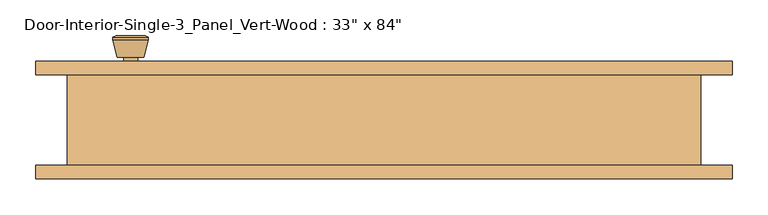
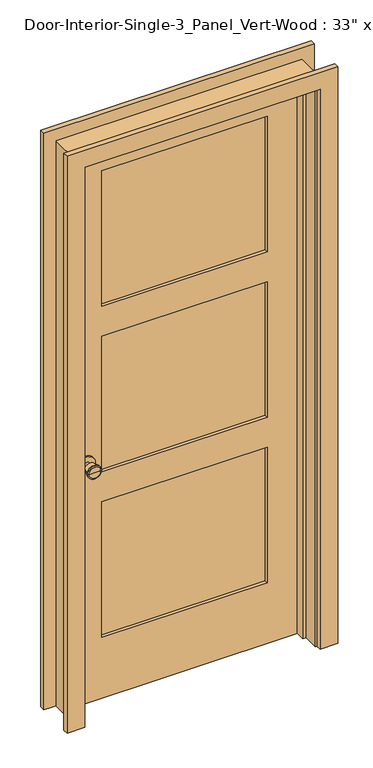
"""IFC4 building model written with IfcOpenShell, lengths in millimetres: door geometry."""

from ifc_helpers import new_model, si_unit, point, frame, frame_2d, origin, place, context, project, spatial, polyline, circle_curve, trimmed, segment, composite_curve, outline, extrude, faceted_brep, source, transform, mapped, element, save
from ifc_brep_helpers import plane_surface, cylinder_surface, revolved_surface, advanced_brep


def door_14766595(model_context):
    return source(origin(), model_context, "Body", "SolidModel", [
        advanced_brep(
        [(-355.6, 19.4, 914.4), (-345.6, 19.4, 914.4), (-365.6, 19.4, 914.4), (-335.1241324, -29.6, 914.4), (-355.6, -29.6, 914.4), (-376.0758676, -29.6, 914.4), (-330.6, -27.7721319, 914.4), (-380.6, -27.7721319, 914.4), (-330.6, -24.3084537, 914.4), (-380.6, -24.3084537, 914.4), (-336.963764, 0.4, 914.4), (-374.236236, 0.4, 914.4), (-345.6, 0.4, 914.4), (-365.6, 0.4, 914.4)],
        [
            (0, 1),
            (1, 2, circle_curve(frame((-355.6, 19.4, 914.4), z_axis=(0.0, 1.0, 0.0), x_axis=(-1.0, 0.0, 0.0)), 10.0)),
            (2, 0),
            (2, 1, circle_curve(frame((-355.6, 19.4, 914.4), z_axis=(0.0, 1.0, 0.0), x_axis=(-1.0, 0.0, 0.0)), 10.0)),
            (3, 4),
            (4, 5),
            (5, 3, circle_curve(frame((-355.6, -29.6, 914.4), z_axis=(0.0, -1.0, 0.0), x_axis=(-1.0, 0.0, 0.0)), 20.4758676)),
            (3, 5, circle_curve(frame((-355.6, -29.6, 914.4), z_axis=(0.0, -1.0, 0.0), x_axis=(-1.0, 0.0, 0.0)), 20.4758676)),
            (6, 3),
            (5, 7),
            (7, 6, circle_curve(frame((-355.6, -27.7721319, 914.4), z_axis=(0.0, -1.0, 0.0), x_axis=(-1.0, 0.0, 0.0)), 25.0)),
            (6, 7, circle_curve(frame((-355.6, -27.7721319, 914.4), z_axis=(0.0, -1.0, 0.0), x_axis=(-1.0, 0.0, 0.0)), 25.0)),
            (8, 6),
            (7, 9),
            (9, 8, circle_curve(frame((-355.6, -24.3084537, 914.4), z_axis=(0.0, -1.0, 0.0), x_axis=(-1.0, 0.0, 0.0)), 25.0)),
            (8, 9, circle_curve(frame((-355.6, -24.3084537, 914.4), z_axis=(0.0, -1.0, 0.0), x_axis=(-1.0, 0.0, 0.0)), 25.0)),
            (10, 8),
            (9, 11),
            (11, 10, circle_curve(frame((-355.6, 0.4, 914.4), z_axis=(0.0, -1.0, 0.0), x_axis=(-1.0, 0.0, 0.0)), 18.636236)),
            (10, 11, circle_curve(frame((-355.6, 0.4, 914.4), z_axis=(0.0, -1.0, 0.0), x_axis=(-1.0, 0.0, 0.0)), 18.636236)),
            (12, 10),
            (11, 13),
            (13, 12, circle_curve(frame((-355.6, 0.4, 914.4), z_axis=(0.0, -1.0, 0.0), x_axis=(-1.0, 0.0, 0.0)), 10.0)),
            (12, 13, circle_curve(frame((-355.6, 0.4, 914.4), z_axis=(0.0, -1.0, 0.0), x_axis=(-1.0, 0.0, 0.0)), 10.0)),
            (1, 12),
            (13, 2),
        ],
        [
            plane_surface(frame((-355.6, 19.4, 914.4), z_axis=(0.0, 1.0, 0.0), x_axis=(-1.0, 0.0, 0.0))),
            plane_surface(frame((-355.6, -29.6, 914.4), z_axis=(0.0, -1.0, 0.0), x_axis=(-1.0, 0.0, 0.0))),
            revolved_surface(polyline([(-376.0758676, -29.6, 914.4), (-380.6, -27.7721319, 914.4)]), (-355.6, 19.4, 914.4), (0.0, 1.0, 0.0)),
            cylinder_surface(frame((-355.6, 19.4, 914.4), z_axis=(0.0, 1.0, 0.0), x_axis=(-1.0, 0.0, 0.0)), 25.0),
            revolved_surface(polyline([(-380.6, -24.3084537, 914.4), (-374.236236, 0.4, 914.4)]), (-355.6, 19.4, 914.4), (0.0, 1.0, 0.0)),
            plane_surface(frame((-355.6, 0.4, 914.4), z_axis=(0.0, 1.0, 0.0), x_axis=(-1.0, 0.0, 0.0))),
            cylinder_surface(frame((-355.6, 19.4, 914.4), z_axis=(0.0, 1.0, 0.0), x_axis=(-1.0, 0.0, 0.0)), 10.0),
        ],
        [
            (0, [[1, 2, 3]]),
            (0, [[-3, 4, -1]]),
            (1, [[5, 6, 7]]),
            (1, [[-6, -5, 8]]),
            (2, [[9, -7, 10, 11]]),
            (2, [[-10, -8, -9, 12]]),
            (3, [[13, -11, 14, 15]]),
            (3, [[-14, -12, -13, 16]]),
            (4, [[17, -15, 18, 19]]),
            (4, [[-18, -16, -17, 20]]),
            (5, [[21, -19, 22, 23]]),
            (5, [[-22, -20, -21, 24]]),
            (6, [[25, -23, 26, -2]]),
            (6, [[-26, -24, -25, -4]]),
        ],
    ),
        extrude(outline(composite_curve([segment(trimmed(circle_curve(frame_2d((914.4, -355.6)), 30.0), [point((914.4, -385.6))], [point((914.4, -325.6))], False, "CARTESIAN"), True, "CONTINUOUS"), segment(trimmed(circle_curve(frame_2d((914.4, -355.6)), 30.0), [point((914.4, -325.6))], [point((914.4, -385.6))], False, "CARTESIAN"), True, "CONTINUOUS")], self_intersect=False)), frame((0.0, 19.4, 0.0), z_axis=(0.0, 1.0, 0.0), x_axis=(0.0, 0.0, 1.0)), (0.0, 0.0, 1.0), 6.0),
        advanced_brep(
        [(-355.6, 66.325, 914.4), (-365.6, 66.325, 914.4), (-345.6, 66.325, 914.4), (-335.1241324, 115.325, 914.4), (-376.0758676, 115.325, 914.4), (-355.6, 115.325, 914.4), (-330.6, 113.4971319, 914.4), (-380.6, 113.4971319, 914.4), (-330.6, 110.0334537, 914.4), (-380.6, 110.0334537, 914.4), (-336.963764, 85.325, 914.4), (-374.236236, 85.325, 914.4), (-345.6, 85.325, 914.4), (-365.6, 85.325, 914.4)],
        [
            (0, 1),
            (1, 2, circle_curve(frame((-355.6, 66.325, 914.4), z_axis=(0.0, -1.0, 0.0), x_axis=(-1.0, 0.0, 0.0)), 10.0)),
            (2, 0),
            (2, 1, circle_curve(frame((-355.6, 66.325, 914.4), z_axis=(0.0, -1.0, 0.0), x_axis=(-1.0, 0.0, 0.0)), 10.0)),
            (3, 4, circle_curve(frame((-355.6, 115.325, 914.4), z_axis=(0.0, 1.0, 0.0), x_axis=(-1.0, 0.0, 0.0)), 20.4758676)),
            (4, 5),
            (5, 3),
            (4, 3, circle_curve(frame((-355.6, 115.325, 914.4), z_axis=(0.0, 1.0, 0.0), x_axis=(-1.0, 0.0, 0.0)), 20.4758676)),
            (6, 7, circle_curve(frame((-355.6, 113.4971319, 914.4), z_axis=(0.0, 1.0, 0.0), x_axis=(-1.0, 0.0, 0.0)), 25.0)),
            (7, 4),
            (3, 6),
            (7, 6, circle_curve(frame((-355.6, 113.4971319, 914.4), z_axis=(0.0, 1.0, 0.0), x_axis=(-1.0, 0.0, 0.0)), 25.0)),
            (8, 9, circle_curve(frame((-355.6, 110.0334537, 914.4), z_axis=(0.0, 1.0, 0.0), x_axis=(-1.0, 0.0, 0.0)), 25.0)),
            (9, 7),
            (6, 8),
            (9, 8, circle_curve(frame((-355.6, 110.0334537, 914.4), z_axis=(0.0, 1.0, 0.0), x_axis=(-1.0, 0.0, 0.0)), 25.0)),
            (10, 11, circle_curve(frame((-355.6, 85.325, 914.4), z_axis=(0.0, 1.0, 0.0), x_axis=(-1.0, 0.0, 0.0)), 18.636236)),
            (11, 9),
            (8, 10),
            (11, 10, circle_curve(frame((-355.6, 85.325, 914.4), z_axis=(0.0, 1.0, 0.0), x_axis=(-1.0, 0.0, 0.0)), 18.636236)),
            (12, 13, circle_curve(frame((-355.6, 85.325, 914.4), z_axis=(0.0, 1.0, 0.0), x_axis=(-1.0, 0.0, 0.0)), 10.0)),
            (13, 11),
            (10, 12),
            (13, 12, circle_curve(frame((-355.6, 85.325, 914.4), z_axis=(0.0, 1.0, 0.0), x_axis=(-1.0, 0.0, 0.0)), 10.0)),
            (1, 13),
            (12, 2),
        ],
        [
            plane_surface(frame((-355.6, 66.325, 914.4), z_axis=(0.0, -1.0, 0.0), x_axis=(-1.0, 0.0, 0.0))),
            plane_surface(frame((-355.6, 115.325, 914.4), z_axis=(0.0, 1.0, 0.0), x_axis=(-1.0, 0.0, 0.0))),
            revolved_surface(polyline([(-376.0758676, 115.325, 914.4), (-380.6, 113.4971319, 914.4)]), (-355.6, 66.325, 914.4), (0.0, -1.0, 0.0)),
            cylinder_surface(frame((-355.6, 66.325, 914.4), z_axis=(0.0, -1.0, 0.0), x_axis=(-1.0, 0.0, 0.0)), 25.0),
            revolved_surface(polyline([(-380.6, 110.0334537, 914.4), (-374.236236, 85.325, 914.4)]), (-355.6, 66.325, 914.4), (0.0, -1.0, 0.0)),
            plane_surface(frame((-355.6, 85.325, 914.4), z_axis=(0.0, -1.0, 0.0), x_axis=(-1.0, 0.0, 0.0))),
            cylinder_surface(frame((-355.6, 66.325, 914.4), z_axis=(0.0, -1.0, 0.0), x_axis=(-1.0, 0.0, 0.0)), 10.0),
        ],
        [
            (0, [[1, 2, 3]]),
            (0, [[-3, 4, -1]]),
            (1, [[5, 6, 7]]),
            (1, [[8, -7, -6]]),
            (2, [[9, 10, -5, 11]]),
            (2, [[12, -11, -8, -10]]),
            (3, [[13, 14, -9, 15]]),
            (3, [[16, -15, -12, -14]]),
            (4, [[17, 18, -13, 19]]),
            (4, [[20, -19, -16, -18]]),
            (5, [[21, 22, -17, 23]]),
            (5, [[24, -23, -20, -22]]),
            (6, [[-2, 25, -21, 26]]),
            (6, [[-4, -26, -24, -25]]),
        ],
    ),
        extrude(outline(composite_curve([segment(trimmed(circle_curve(frame_2d((914.4, -355.6)), 30.0), [point((914.4, -385.6))], [point((914.4, -325.6))], False, "CARTESIAN"), True, "CONTINUOUS"), segment(trimmed(circle_curve(frame_2d((914.4, -355.6)), 30.0), [point((914.4, -325.6))], [point((914.4, -385.6))], False, "CARTESIAN"), True, "CONTINUOUS")], self_intersect=False)), frame((0.0, 60.325, 0.0), z_axis=(0.0, 1.0, 0.0), x_axis=(0.0, 0.0, 1.0)), (0.0, 0.0, 1.0), 6.0),
        faceted_brep([(444.5, 60.325, 0.0), (444.5, -66.675, 0.0), (419.1, -66.675, 0.0), (419.1, -9.525, 0.0), (406.4, -9.525, 0.0), (406.4, 25.4, 0.0), (419.1, 25.4, 0.0), (419.1, 60.325, 0.0), (444.5, 60.325, 2159.0), (444.5, -66.675, 2159.0), (-444.5, -66.675, 2159.0), (-444.5, -66.675, 0.0), (-419.1, -66.675, 0.0), (-419.1, -66.675, 2133.6), (419.1, -66.675, 2133.6), (419.1, -9.525, 2133.6), (-419.1, -9.525, 2133.6), (-419.1, -9.525, 0.0), (-406.4, -9.525, 0.0), (-406.4, -9.525, 2120.9), (406.4, -9.525, 2120.9), (406.4, 25.4, 2120.9), (-406.4, 25.4, 2120.9), (-406.4, 25.4, 0.0), (-419.1, 25.4, 0.0), (-419.1, 25.4, 2133.6), (419.1, 25.4, 2133.6), (419.1, 60.325, 2133.6), (-419.1, 60.325, 2133.6), (-419.1, 60.325, 0.0), (-444.5, 60.325, 0.0), (-444.5, 60.325, 2159.0)], [[[0, 1, 2, 3, 4, 5, 6, 7]], [[1, 0, 8, 9]], [[2, 1, 9, 10, 11, 12, 13, 14]], [[3, 2, 14, 15]], [[4, 3, 15, 16, 17, 18, 19, 20]], [[5, 4, 20, 21]], [[6, 5, 21, 22, 23, 24, 25, 26]], [[7, 6, 26, 27]], [[0, 7, 27, 28, 29, 30, 31, 8]], [[9, 8, 31, 10]], [[15, 14, 13, 16]], [[21, 20, 19, 22]], [[27, 26, 25, 28]], [[30, 29, 24, 23, 18, 17, 12, 11]], [[10, 31, 30, 11]], [[16, 13, 12, 17]], [[22, 19, 18, 23]], [[28, 25, 24, 29]]]),
        extrude(outline(polyline([(2133.6, -419.1), (0.0, -419.1), (0.0, 419.1), (2133.6, 419.1), (2133.6, -419.1)]), holes=[polyline([(2014.5375, -298.45), (2014.5375, 298.45), (1496.4833333, 298.45), (1496.4833333, -298.45), (2014.5375, -298.45)]), polyline([(749.8291667, -298.45), (749.8291667, 298.45), (231.775, 298.45), (231.775, -298.45), (749.8291667, -298.45)]), polyline([(1382.1833333, -298.45), (1382.1833333, 298.45), (864.1291667, 298.45), (864.1291667, -298.45), (1382.1833333, -298.45)])]), frame((0.0, 25.4, 0.0), z_axis=(0.0, 1.0, 0.0), x_axis=(0.0, 0.0, 1.0)), (0.0, 0.0, 1.0), 34.925),
        extrude(outline(polyline([(298.45, 37.0416667), (-298.45, 37.0416667), (-298.45, 48.6833333), (298.45, 48.6833333), (298.45, 37.0416667)])), frame((0.0, 0.0, 1496.4833333), z_axis=(0.0, 0.0, 1.0), x_axis=(1.0, 0.0, 0.0)), (0.0, 0.0, 1.0), 518.0541667),
        extrude(outline(polyline([(298.45, 37.0416667), (-298.45, 37.0416667), (-298.45, 48.6833333), (298.45, 48.6833333), (298.45, 37.0416667)])), frame((0.0, 0.0, 231.775), z_axis=(0.0, 0.0, 1.0), x_axis=(1.0, 0.0, 0.0)), (0.0, 0.0, 1.0), 518.0541667),
        extrude(outline(polyline([(298.45, 37.0416667), (-298.45, 37.0416667), (-298.45, 48.6833333), (298.45, 48.6833333), (298.45, 37.0416667)])), frame((0.0, 0.0, 864.1291667), z_axis=(0.0, 0.0, 1.0), x_axis=(1.0, 0.0, 0.0)), (0.0, 0.0, 1.0), 518.0541667),
        extrude(outline(polyline([(0.0, 425.45), (0.0, 488.95), (2203.45, 488.95), (2203.45, -488.95), (0.0, -488.95), (0.0, -425.45), (2139.95, -425.45), (2139.95, 425.45), (0.0, 425.45)])), frame((0.0, 60.325, 0.0), z_axis=(0.0, 1.0, 0.0), x_axis=(0.0, 0.0, 1.0)), (0.0, 0.0, 1.0), 19.05),
        extrude(outline(polyline([(0.0, 425.45), (0.0, 488.95), (2203.45, 488.95), (2203.45, -488.95), (0.0, -488.95), (0.0, -425.45), (2139.95, -425.45), (2139.95, 425.45), (0.0, 425.45)])), frame((0.0, -85.725, 0.0), z_axis=(0.0, 1.0, 0.0), x_axis=(0.0, 0.0, 1.0)), (0.0, 0.0, 1.0), 19.05),
    ])


if __name__ == "__main__":
    model = new_model("IFC4")
    model_context = context("Model", 3, world=origin())
    ifc_project = project(units=[si_unit("LENGTHUNIT", "METRE", prefix="MILLI")], contexts=[model_context])
    site = spatial("IfcSite", under=ifc_project)
    building = spatial("IfcBuilding", under=site)
    placement = place(None, origin())
    door_shape = door_14766595(model_context)
    element("IfcDoor", 1, ObjectType="Door-Interior-Single-3_Panel_Vert-Wood : 33\" x 84\"", at=placement, inside=building, context=model_context, shape_type="MappedRepresentation", body=[
        mapped(door_shape, transform((0.0, 0.0, 0.0), x_axis=(1.0, 0.0, 0.0), y_axis=(0.0, 1.0, 0.0), z_axis=(0.0, 0.0, 1.0))),
    ])
    save(model, "model.ifc")

# Revit data of these elements
# Type "Door-Interior-Single-3_Panel_Vert-Wood : 33\" x 84\""
#   Type Mark = "11"
#   Assembly Code = "C1020300"
#   Analytic Construction = "Wooden"
#   Top Rail = 0' - 4 11/16"
#   Thickness = 0' - 1 3/8"
#   Thermal Resistance (R) = 2.5876 (h·ft²·°F)/BTU
#   Swing Angle [instance default] = 90.00°
#   Stiles = 0' - 4 3/4"
#   Rough Width = 2' - 11"
#   Rough Height = 7' - 1"
#   Intermediate Rail = 0' - 4 1/2"
#   Height = 7' - 0"
#   Width = 2' - 9"
#   Heat Transfer Coefficient (U) = 0.3865 BTU/(h·ft²·°F)
#   Bottom Rail = 0' - 9 1/8"
#   Trim Material = Cherry
#   Panel Material = Cherry
#   Frame Material = Cherry
#   Door Handle Material = Aluminum
#   Visual Light Transmittance = 0
#   Solar Heat Gain Coefficient = 0
#   Wall Closure = (empty or 0)
#   Function = (empty or 0)
# Element 1 (IfcDoor, "Door-Interior-Single-3_Panel_Vert-Wood : 33\" x 84\"")
#   Materials on its faces: "Cherry", "Aluminum"
# Materials
#   "Cherry": class "Wood", colour RGB 226 177 128, transparency 0, Description = "Prunus Serotina", Cost = 0
#   "Aluminum": class "Metal", colour RGB 247 247 247, transparency 0, Description = "Aluminum 6061", Cost = 0
